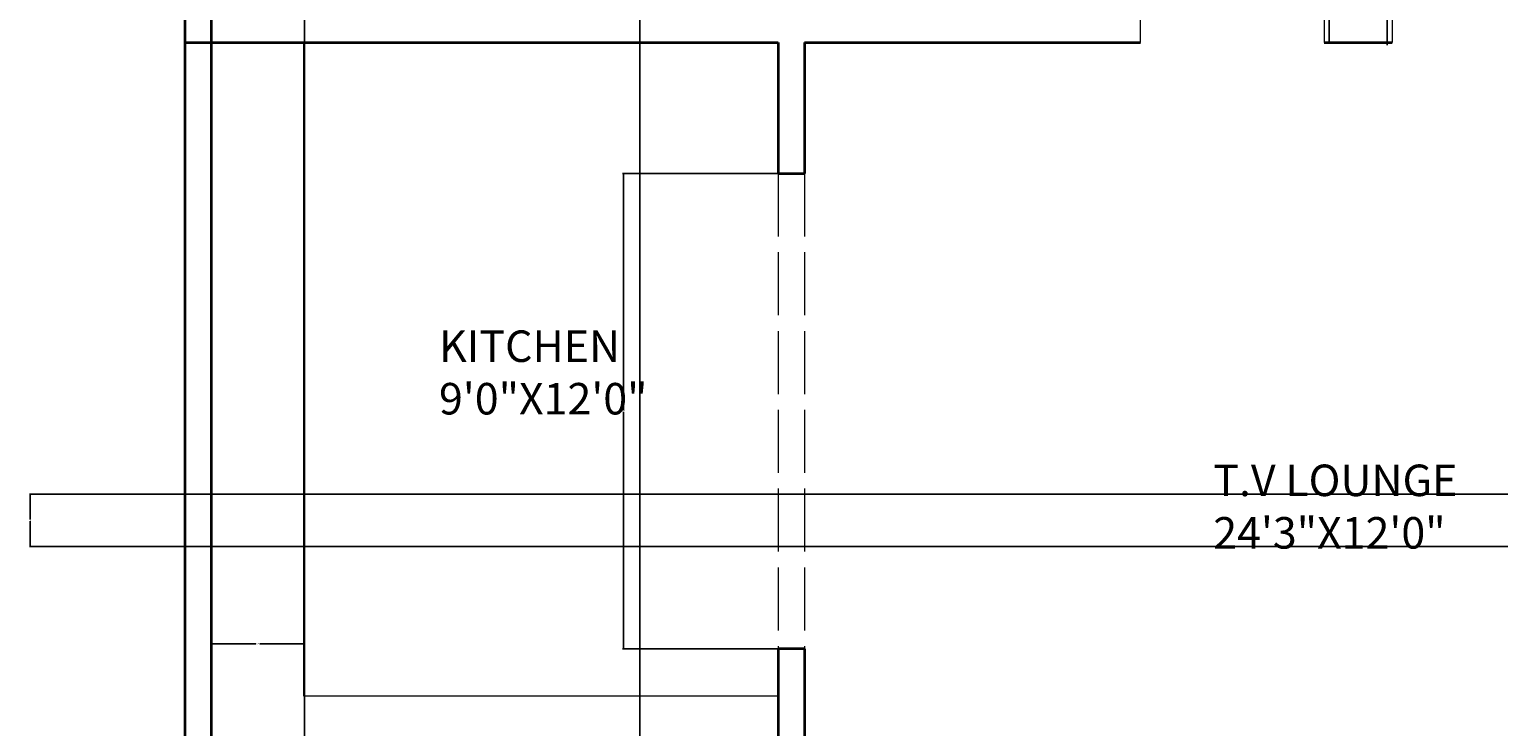
# Model space of a CAD drawing. Units: inches. Extents: x 40921 to 41493, y 89872 to 90511.
# Tile 2 of 4: x 40922 to 41201, y 90120 to 90253. Entities that reach past the tile are written whole.
import ezdxf

# ---------------------------------------------------------------- set-up
doc = ezdxf.new("R2010")
doc.units = ezdxf.units.IN
doc.header["$MEASUREMENT"] = 0
doc.linetypes.add('ACAD_ISO02W100', pattern=[15, 12, -3])
for name, color, linetype, lineweight in [('A-ANNO-DIMS', 2, 'Continuous', 18), ('A-AREA-IDEN', 7, 'Continuous', 18), ('A-DOOR', 3, 'Continuous', 20), ('A-FLOR-CASE', 8, 'Continuous', 18), ('A-WALL', 7, 'Continuous', 35), ('A-WALL-OVHD', 8, 'ACAD_ISO02W100', 13)]:
    doc.layers.add(name, color=color, linetype=linetype, lineweight=lineweight)
doc.styles.get("Standard").update_dxf_attribs({"font": 'arial.ttf'})
doc.dimstyles.get("Standard").update_dxf_attribs({"dimtxt": 0.18, "dimasz": 0.18, "dimexe": 0.18, "dimexo": 0.0625, "dimgap": 0.09, "dimtad": 0, "dimtih": 1, "dimtoh": 1, "dimdec": 4, "dimzin": 0, "dimdsep": 46, "dimtxsty": 'Standard', "dimcen": 0.09, "dimadec": 0, "dimazin": 0, "dimtfac": 1, "dimtdec": 4, "dimtofl": 0, "dimtmove": 0, "dimatfit": 3, "dimfxl": 1, "dimtolj": 1, "dimtzin": 0, "dimarcsym": 0})

# ---------------------------------------------------------------- blocks, each defined once
blk = doc.blocks.new('DOOR-SWING-36IN')
for p, q in [((3, 0), (3, 36)), ((3, 36), (3, 0)), ((4, 36), (4, 0)), ((39, 0), (39, 5)), ((0, 0), (3, 0)), ((3, 0), (4, 0))]:
    blk.add_line(p, q)
blk.add_arc((3, -0.4), 36.4, 8.5358, 90)
blk = doc.blocks.new('*D25')
at = {"layer": 'A-ANNO-DIMS', "color": 0, "lineweight": -2, "transparency": 16777216}
for p, q in [((40973.9, 90106.69), (40973.9, 90511.26)), ((40974.08, 90511.08), (41005.48, 90511.08)), ((41037.63, 90511.08), (41006.23, 90511.08)), ((41037.81, 90106.69), (41037.81, 90511.26))]:
    blk.add_line(p, q, dxfattribs=at)
at = {"layer": 'A-ANNO-DIMS', "color": 0, "transparency": 16777216}
for points in [[(40974.08, 90511.11), (40974.08, 90511.05), (40973.9, 90511.08)], [(41037.63, 90511.11), (41037.63, 90511.05), (41037.81, 90511.08)]]:
    blk.add_solid(points, dxfattribs=at)
at = {"layer": 'Defpoints', "color": 0, "transparency": 16777216}
for p in [(41037.81, 90511.08), (40973.9, 90106.63), (41037.81, 90106.63)]:
    blk.add_point(p, dxfattribs=at)
at = {"layer": 'A-ANNO-DIMS', "color": 0, "transparency": 16777216, "insert": (41005.85, 90511.08), "char_height": 0.18, "attachment_point": 5}
blk.add_mtext('\\A1;63.91', dxfattribs=at)
blk = doc.blocks.new('*D26')
at = {"layer": 'A-ANNO-DIMS', "color": 0, "lineweight": -2, "transparency": 16777216}
for p, q in [((40956.15, 90106.69), (40956.15, 90136.26)), ((40956.33, 90136.08), (40964.64, 90136.08)), ((40973.72, 90136.08), (40965.41, 90136.08)), ((40973.9, 90106.69), (40973.9, 90136.26))]:
    blk.add_line(p, q, dxfattribs=at)
at = {"layer": 'A-ANNO-DIMS', "color": 0, "transparency": 16777216}
for points in [[(40956.33, 90136.11), (40956.33, 90136.05), (40956.15, 90136.08)], [(40973.72, 90136.11), (40973.72, 90136.05), (40973.9, 90136.08)]]:
    blk.add_solid(points, dxfattribs=at)
at = {"layer": 'Defpoints', "color": 0, "transparency": 16777216}
for p in [(40973.9, 90136.08), (40956.15, 90106.63), (40973.9, 90106.63)]:
    blk.add_point(p, dxfattribs=at)
at = {"layer": 'A-ANNO-DIMS', "color": 0, "transparency": 16777216, "insert": (40965.02, 90136.08), "char_height": 0.18, "attachment_point": 5}
blk.add_mtext('\\A1;17.75', dxfattribs=at)
blk = doc.blocks.new('*D28')
at = {"layer": 'A-ANNO-DIMS', "color": 0, "lineweight": -2, "transparency": 16777216}
for p, q in [((41309.09, 90164.63), (40921.52, 90164.63)), ((40921.7, 90164.45), (40921.7, 90159.81)), ((40921.7, 90154.81), (40921.7, 90159.45)), ((41309.09, 90154.63), (40921.52, 90154.63))]:
    blk.add_line(p, q, dxfattribs=at)
at = {"layer": 'A-ANNO-DIMS', "color": 0, "transparency": 16777216}
for points in [[(40921.67, 90164.45), (40921.73, 90164.45), (40921.7, 90164.63)], [(40921.67, 90154.81), (40921.73, 90154.81), (40921.7, 90154.63)]]:
    blk.add_solid(points, dxfattribs=at)
at = {"layer": 'Defpoints', "color": 0, "transparency": 16777216}
for p in [(40921.7, 90164.63), (41309.15, 90164.63), (41309.15, 90154.63)]:
    blk.add_point(p, dxfattribs=at)
at = {"layer": 'A-ANNO-DIMS', "color": 0, "transparency": 16777216, "insert": (40921.7, 90159.63), "char_height": 0.18, "attachment_point": 5}
blk.add_mtext('\\A1;10', dxfattribs=at)
blk = doc.blocks.new('*D30')
at = {"layer": 'A-ANNO-DIMS', "color": 0, "lineweight": -2, "transparency": 16777216}
for p, q in [((41064.09, 90225.67), (41034.52, 90225.67)), ((41034.7, 90225.49), (41034.7, 90180.59)), ((41034.7, 90135.33), (41034.7, 90180.23)), ((41064.09, 90135.15), (41034.52, 90135.15))]:
    blk.add_line(p, q, dxfattribs=at)
at = {"layer": 'A-ANNO-DIMS', "color": 0, "transparency": 16777216}
for points in [[(41034.67, 90225.49), (41034.73, 90225.49), (41034.7, 90225.67)], [(41034.67, 90135.33), (41034.73, 90135.33), (41034.7, 90135.15)]]:
    blk.add_solid(points, dxfattribs=at)
at = {"layer": 'Defpoints', "color": 0, "transparency": 16777216}
for p in [(41034.7, 90225.67), (41064.15, 90225.67), (41064.15, 90135.15)]:
    blk.add_point(p, dxfattribs=at)
at = {"layer": 'A-ANNO-DIMS', "color": 0, "transparency": 16777216, "insert": (41034.7, 90180.41), "char_height": 0.18, "attachment_point": 5}
blk.add_mtext('\\A1;90.52', dxfattribs=at)
blk = doc.blocks.new('*D46')
at = {"layer": 'A-ANNO-DIMS', "color": 0, "lineweight": -2, "transparency": 16777216}
for p, q in [((41218.16, 90294.36), (41204.02, 90277.95)), ((41218.34, 90294.36), (41218.16, 90294.36)), ((41180.06, 90250.23), (41180.24, 90250.23)), ((41180.15, 90250.14), (41180.15, 90250.32))]:
    blk.add_line(p, q, dxfattribs=at)
at = {"layer": 'A-ANNO-DIMS', "color": 0, "transparency": 16777216}
blk.add_solid([(41204, 90277.97), (41204.04, 90277.93), (41203.9, 90277.81)], dxfattribs=at)
at = {"layer": 'Defpoints', "color": 0, "transparency": 16777216}
for p in [(41203.9, 90277.81), (41180.15, 90250.23)]:
    blk.add_point(p, dxfattribs=at)
at = {"layer": 'A-ANNO-DIMS', "color": 0, "transparency": 16777216, "insert": (41218.94, 90294.36), "char_height": 0.18, "attachment_point": 5}
blk.add_mtext('\\A1;2X R36.4', dxfattribs=at)

msp = doc.modelspace()

# ---------------------------------------------------------------- linework, layer by layer
at = {"layer": 'A-FLOR-CASE'}
for p, q in [((40973.7135, 90250.6306), (40973.7135, 90126.2229)), ((40973.7135, 90126.2229), (40973.7135, 90126.2229)), ((40973.7135, 90126.2229), (41064.1503, 90126.2229))]:
    msp.add_line(p, q, dxfattribs=at)
at = {"layer": 'A-WALL'}
for p, q in [((40951.1503, 90481.6306), (40951.1503, 89901.6306)), ((40956.1503, 90476.6306), (40956.1503, 90106.6306)), ((40951.1503, 90250.6306), (41064.1503, 90250.6306)), ((41064.1503, 90250.6306), (41064.1503, 90225.6679)), ((41069.1503, 90250.6306), (41069.1503, 90225.6679)), ((41069.1503, 90250.6306), (41133.1503, 90250.6306)), ((41168.1503, 90250.6306), (41181.1503, 90250.6306)), ((41064.1503, 90225.6679), (41069.1503, 90225.6679)), ((41069.1503, 90135.1497), (41064.1503, 90135.1497)), ((41064.1503, 90135.1497), (41064.1503, 90106.6306)), ((41069.1503, 90135.1497), (41069.1503, 90106.6306))]:
    msp.add_line(p, q, dxfattribs=at)
at = {"layer": 'A-WALL-OVHD'}
for p, q in [((41064.1503, 90225.6679), (41064.1503, 90135.1497)), ((41069.1503, 90225.6679), (41069.1503, 90135.1497))]:
    msp.add_line(p, q, dxfattribs=at)

# ---------------------------------------------------------------- block references
at = {"layer": 'A-DOOR', "extrusion": (0, 0, -1), "zscale": -1}
msp.add_blockref('DOOR-SWING-36IN', (-41172.1506, 90250.631), dxfattribs=at)
at = {"layer": 'A-DOOR'}
msp.add_blockref('DOOR-SWING-36IN', (41177.15, 90250.631), dxfattribs=at)

# ---------------------------------------------------------------- texts
at = {"layer": 'A-AREA-IDEN', "char_height": 6, "attachment_point": 1}
for s, width, insert in [('KITCHEN\\P9\'0"X12\'0"', 75.44991, (40999.5518, 90195.7884)), ('T.V LOUNGE\\P24\'3"X12\'0"', 85.047977, (41147.0369, 90170.2395))]:
    msp.add_mtext_dynamic_manual_height_columns(s, width=width, gutter_width=1, heights=[0], dxfattribs=dict(at, insert=insert))

# ---------------------------------------------------------------- dimensions: what is measured, and where the dimension line sits
at = {"layer": 'A-ANNO-DIMS'}
for base, p1, p2, picture, middle in [((41037.8072, 90511.0806), (40973.8989, 90106.6306), (41037.8072, 90106.6306), '*D25', (41005.8531, 90511.0806)), ((40973.8989, 90136.0806), (40956.1503, 90106.6306), (40973.8989, 90106.6306), '*D26', (40965.0246, 90136.0806))]:
    dim = msp.add_linear_dim(base=base, p1=p1, p2=p2, dimstyle='Standard', override={"dimdec": 2, "dimlfac": 1, "dimrnd": 0, "dimzin": 0, "dimdsep": 46, "dimlunit": 2}, dxfattribs=at)
    dim.commit()
    dim.dimension.update_dxf_attribs({"geometry": picture, "text_midpoint": middle})
dim = msp.add_radius_dim(center=(41180.1503, 90250.2274), mpoint=(41203.9039, 90277.8129), text='2X <>', dimstyle='Standard', override={"dimdec": 1, "dimlfac": 1, "dimrnd": 0, "dimzin": 0, "dimdsep": 46, "dimlunit": 2}, dxfattribs=at)
dim.commit()
dim.dimension.update_dxf_attribs({"geometry": '*D46', "text_midpoint": (41218.9406, 90294.3642), "dimtype": 164})
for base, p1, p2, override, picture, middle in [((41034.7003, 90225.6679), (41064.1503, 90135.1497), (41064.1503, 90225.6679), {"dimdec": 2, "dimlfac": 1, "dimrnd": 0, "dimzin": 0, "dimdsep": 46, "dimlunit": 2}, '*D30', (41034.7003, 90180.4088)), ((40921.7003, 90164.6306), (41309.1503, 90154.6306), (41309.1503, 90164.6306), {"dimdec": 0, "dimlfac": 1, "dimrnd": 0, "dimzin": 0, "dimdsep": 46, "dimlunit": 2}, '*D28', (40921.7003, 90159.6306))]:
    dim = msp.add_linear_dim(base=base, p1=p1, p2=p2, angle=90, dimstyle='Standard', override=override, dxfattribs=at)
    dim.commit()
    dim.dimension.update_dxf_attribs({"geometry": picture, "text_midpoint": middle})

doc.saveas('drawing.dxf')
